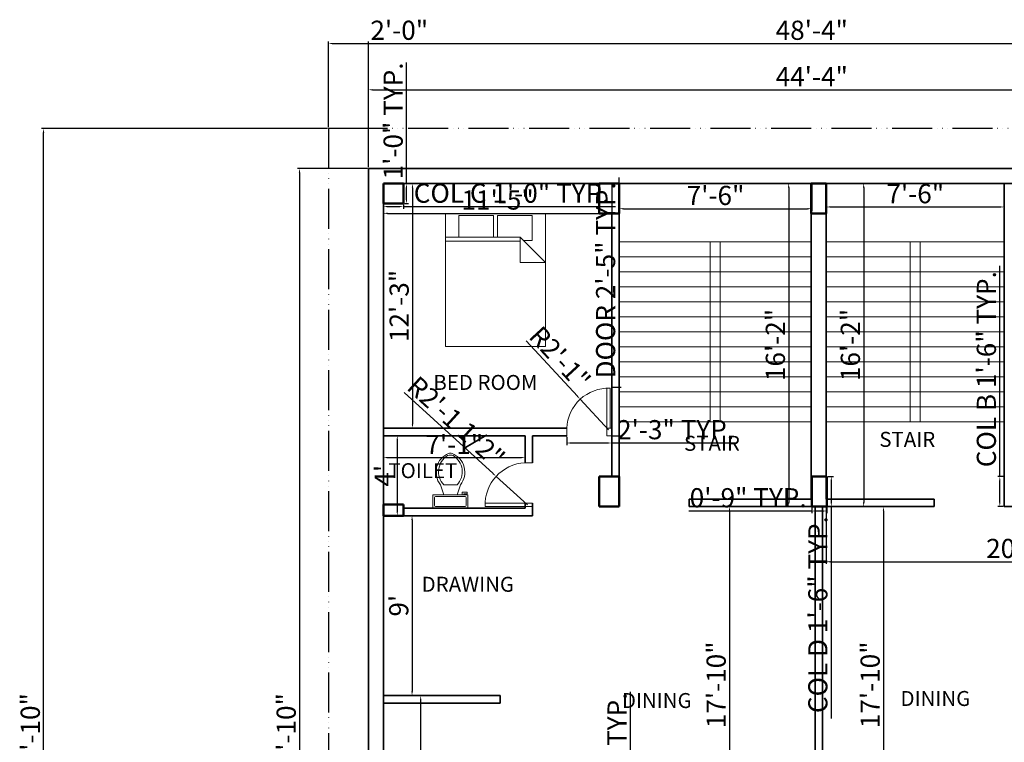
# Model space of a CAD drawing. Units: inches. Extents: x 2680 to 3617, y 1720 to 2823.
# Tile 3 of 4: x 2680 to 3270, y 2380 to 2814. Entities that reach past the tile are written whole.
import ezdxf

# ---------------------------------------------------------------- set-up
doc = ezdxf.new("R2010")
doc.units = ezdxf.units.IN
doc.linetypes.add('ACAD_ISO06W100', pattern=[36, 24, -3, 0, -3, 0, -3, 0, -3])
for name, color, linetype, lineweight in [('A-ANNO-DIMS', 2, 'Continuous', 18), ('A-AREA-IDEN', 244, 'Continuous', 18), ('A-COLS', 1, 'Continuous', 50), ('A-DOOR', 4, 'Continuous', 18), ('A-FLOR-FIXT', 9, 'Continuous', 18), ('A-FLOR-STRS', 7, 'Continuous', 18), ('A-FURN', 8, 'Continuous', 18), ('A-WALL', 7, 'Continuous', 35), ('C-PROP', 6, 'ACAD_ISO06W100', 25)]:
    doc.layers.add(name, color=color, linetype=linetype, lineweight=lineweight)
doc.styles.get("Standard").update_dxf_attribs({"font": 'arial.ttf'})
doc.dimstyles.new('ISO-25', dxfattribs={"dimtxt": 11.5, "dimasz": 2.5, "dimexe": 1.25, "dimexo": 0.625, "dimtad": 1, "dimdec": 1, "dimlunit": 3, "dimtxsty": 'Standard', "dimcen": 2.5, "dimadec": 0, "dimazin": 0, "dimtfac": 1, "dimtdec": 1, "dimtmove": 0, "dimatfit": 3, "dimfxl": 1, "dimarcsym": 0})

# ---------------------------------------------------------------- blocks, each defined once
blk = doc.blocks.new('*D2')
at = {"layer": 'A-ANNO-DIMS', "color": 0, "lineweight": -2, "transparency": 16777216}
for p, q in [((2898.54, 2715.34), (2916.59, 2715.34)), ((2915.34, 2712.84), (2915.34, 2571)), ((2898.54, 2568.5), (2916.59, 2568.5))]:
    blk.add_line(p, q, dxfattribs=at)
at = {"layer": 'A-ANNO-DIMS', "color": 0, "lineweight": 70, "transparency": 16777216}
for points in [[(2914.92, 2712.84), (2915.76, 2712.84), (2915.34, 2715.34)], [(2914.92, 2571), (2915.76, 2571), (2915.34, 2568.5)]]:
    blk.add_solid(points, dxfattribs=at)
at = {"layer": 'Defpoints', "color": 0, "lineweight": 70, "transparency": 16777216}
for p in [(2897.91, 2715.34), (2897.91, 2568.5), (2915.34, 2568.5)]:
    blk.add_point(p, dxfattribs=at)
at = {"layer": 'A-ANNO-DIMS', "color": 0, "transparency": 16777216, "insert": (2908.84, 2641.92), "char_height": 11.5, "attachment_point": 5, "rotation": 90}
blk.add_mtext('12\'-3"', dxfattribs=at)
blk = doc.blocks.new('*D3')
at = {"layer": 'A-ANNO-DIMS', "color": 0, "lineweight": -2, "transparency": 16777216}
for p, q in [((2897.91, 2714.88), (2897.91, 2696.25)), ((3034.91, 2714.88), (3034.91, 2696.25)), ((2900.41, 2697.5), (3032.41, 2697.5))]:
    blk.add_line(p, q, dxfattribs=at)
at = {"layer": 'A-ANNO-DIMS', "color": 0, "lineweight": 70, "transparency": 16777216}
for points in [[(2900.41, 2697.92), (2900.41, 2697.09), (2897.91, 2697.5)], [(3032.41, 2697.92), (3032.41, 2697.09), (3034.91, 2697.5)]]:
    blk.add_solid(points, dxfattribs=at)
at = {"layer": 'Defpoints', "color": 0, "lineweight": 70, "transparency": 16777216}
for p in [(2897.91, 2715.5), (3034.91, 2715.5), (3034.91, 2697.5)]:
    blk.add_point(p, dxfattribs=at)
at = {"layer": 'A-ANNO-DIMS', "color": 0, "transparency": 16777216, "insert": (2966.41, 2704), "char_height": 11.5, "attachment_point": 5}
blk.add_mtext('11\'-5"', dxfattribs=at)
blk = doc.blocks.new('*D4')
at = {"layer": 'A-ANNO-DIMS', "color": 0, "lineweight": -2, "transparency": 16777216}
for p, q in [((3039.41, 2714.88), (3039.41, 2699.02)), ((3154.91, 2714.88), (3154.91, 2699.02)), ((3041.91, 2700.27), (3152.41, 2700.27))]:
    blk.add_line(p, q, dxfattribs=at)
at = {"layer": 'A-ANNO-DIMS', "color": 0, "lineweight": 70, "transparency": 16777216}
for points in [[(3041.91, 2700.68), (3041.91, 2699.85), (3039.41, 2700.27)], [(3152.41, 2700.68), (3152.41, 2699.85), (3154.91, 2700.27)]]:
    blk.add_solid(points, dxfattribs=at)
at = {"layer": 'Defpoints', "color": 0, "lineweight": 70, "transparency": 16777216}
for p in [(3039.41, 2715.5), (3154.91, 2715.5), (3154.91, 2700.27)]:
    blk.add_point(p, dxfattribs=at)
at = {"layer": 'A-ANNO-DIMS', "color": 0, "transparency": 16777216, "insert": (3097.16, 2706.76), "char_height": 11.5, "attachment_point": 5}
blk.add_mtext('7\'-6"', dxfattribs=at)
blk = doc.blocks.new('*D5')
at = {"layer": 'A-ANNO-DIMS', "color": 0, "lineweight": -2, "transparency": 16777216}
for p, q in [((3163.61, 2714.88), (3163.61, 2700.07)), ((3270.41, 2714.8), (3270.41, 2700.07)), ((3166.11, 2701.32), (3267.91, 2701.32))]:
    blk.add_line(p, q, dxfattribs=at)
at = {"layer": 'A-ANNO-DIMS', "color": 0, "lineweight": 70, "transparency": 16777216}
for points in [[(3166.11, 2701.74), (3166.11, 2700.91), (3163.61, 2701.32)], [(3267.91, 2701.74), (3267.91, 2700.91), (3270.41, 2701.32)]]:
    blk.add_solid(points, dxfattribs=at)
at = {"layer": 'Defpoints', "color": 0, "lineweight": 70, "transparency": 16777216}
for p in [(3163.61, 2715.5), (3270.41, 2715.43), (3270.41, 2701.32)]:
    blk.add_point(p, dxfattribs=at)
at = {"layer": 'A-ANNO-DIMS', "color": 0, "transparency": 16777216, "insert": (3217.01, 2707.82), "char_height": 11.5, "width": 83.0724, "attachment_point": 5}
blk.add_mtext('7\'-6"', dxfattribs=at)
blk = doc.blocks.new('*D6')
at = {"layer": 'A-ANNO-DIMS', "color": 0, "lineweight": -2, "transparency": 16777216}
for p, q in [((3154.29, 2715.5), (3139.79, 2715.5)), ((3141.04, 2713), (3141.04, 2524)), ((3154.29, 2521.5), (3139.79, 2521.5))]:
    blk.add_line(p, q, dxfattribs=at)
at = {"layer": 'A-ANNO-DIMS', "color": 0, "lineweight": 70, "transparency": 16777216}
for points in [[(3140.62, 2713), (3141.46, 2713), (3141.04, 2715.5)], [(3140.62, 2524), (3141.46, 2524), (3141.04, 2521.5)]]:
    blk.add_solid(points, dxfattribs=at)
at = {"layer": 'Defpoints', "color": 0, "lineweight": 70, "transparency": 16777216}
for p in [(3154.91, 2715.5), (3141.04, 2521.5), (3154.91, 2521.5)]:
    blk.add_point(p, dxfattribs=at)
at = {"layer": 'A-ANNO-DIMS', "color": 0, "transparency": 16777216, "insert": (3134.54, 2618.5), "char_height": 11.5, "attachment_point": 5, "rotation": 90}
blk.add_mtext('16\'-2"', dxfattribs=at)
blk = doc.blocks.new('*D7')
at = {"layer": 'A-ANNO-DIMS', "color": 0, "lineweight": -2, "transparency": 16777216}
for p, q in [((3164.24, 2715.5), (3187.29, 2715.5)), ((3186.04, 2713), (3186.04, 2524)), ((3164.24, 2521.5), (3187.29, 2521.5))]:
    blk.add_line(p, q, dxfattribs=at)
at = {"layer": 'A-ANNO-DIMS', "color": 0, "lineweight": 70, "transparency": 16777216}
for points in [[(3185.62, 2713), (3186.45, 2713), (3186.04, 2715.5)], [(3185.62, 2524), (3186.45, 2524), (3186.04, 2521.5)]]:
    blk.add_solid(points, dxfattribs=at)
at = {"layer": 'Defpoints', "color": 0, "lineweight": 70, "transparency": 16777216}
for p in [(3163.61, 2715.5), (3163.61, 2521.5), (3186.04, 2521.5)]:
    blk.add_point(p, dxfattribs=at)
at = {"layer": 'A-ANNO-DIMS', "color": 0, "transparency": 16777216, "insert": (3179.54, 2618.5), "char_height": 11.5, "attachment_point": 5, "rotation": 90}
blk.add_mtext('16\'-2"', dxfattribs=at)
blk = doc.blocks.new('*D10')
at = {"layer": 'A-ANNO-DIMS', "color": 0, "lineweight": -2, "transparency": 16777216}
for p, q in [((2897.91, 2563.38), (2897.91, 2549.63)), ((2982.91, 2563.38), (2982.91, 2549.63)), ((2900.41, 2550.88), (2980.41, 2550.88))]:
    blk.add_line(p, q, dxfattribs=at)
at = {"layer": 'A-ANNO-DIMS', "color": 0, "lineweight": 70, "transparency": 16777216}
for points in [[(2900.41, 2551.3), (2900.41, 2550.46), (2897.91, 2550.88)], [(2980.41, 2551.3), (2980.41, 2550.46), (2982.91, 2550.88)]]:
    blk.add_solid(points, dxfattribs=at)
at = {"layer": 'Defpoints', "color": 0, "lineweight": 70, "transparency": 16777216}
for p in [(2897.91, 2564), (2982.91, 2564), (2982.91, 2550.88)]:
    blk.add_point(p, dxfattribs=at)
at = {"layer": 'A-ANNO-DIMS', "color": 0, "transparency": 16777216, "insert": (2940.41, 2557.28), "char_height": 11.5, "attachment_point": 5}
blk.add_mtext('7\'-1"', dxfattribs=at)
blk = doc.blocks.new('*D11')
at = {"layer": 'A-ANNO-DIMS', "color": 0, "lineweight": -2, "transparency": 16777216}
for p, q in [((2898.54, 2564), (2907.47, 2564)), ((2906.22, 2561.5), (2906.22, 2518.5)), ((2898.54, 2516), (2907.47, 2516))]:
    blk.add_line(p, q, dxfattribs=at)
at = {"layer": 'A-ANNO-DIMS', "color": 0, "lineweight": 70, "transparency": 16777216}
for points in [[(2905.8, 2561.5), (2906.63, 2561.5), (2906.22, 2564)], [(2905.8, 2518.5), (2906.63, 2518.5), (2906.22, 2516)]]:
    blk.add_solid(points, dxfattribs=at)
at = {"layer": 'Defpoints', "color": 0, "lineweight": 70, "transparency": 16777216}
for p in [(2897.91, 2564), (2897.91, 2516), (2906.22, 2516)]:
    blk.add_point(p, dxfattribs=at)
at = {"layer": 'A-ANNO-DIMS', "color": 0, "transparency": 16777216, "insert": (2899.84, 2540), "char_height": 11.5, "attachment_point": 5, "rotation": 90}
blk.add_mtext("4'", dxfattribs=at)
blk = doc.blocks.new('*D15')
at = {"layer": 'A-ANNO-DIMS', "color": 0, "lineweight": -2, "transparency": 16777216}
for p, q in [((2898.54, 2408), (2921.5, 2408)), ((2920.25, 2405.5), (2920.25, 2305.5)), ((2898.54, 2303), (2921.5, 2303))]:
    blk.add_line(p, q, dxfattribs=at)
at = {"layer": 'A-ANNO-DIMS', "color": 0, "lineweight": 70, "transparency": 16777216}
for points in [[(2919.83, 2405.5), (2920.66, 2405.5), (2920.25, 2408)], [(2919.83, 2305.5), (2920.66, 2305.5), (2920.25, 2303)]]:
    blk.add_solid(points, dxfattribs=at)
at = {"layer": 'Defpoints', "color": 0, "lineweight": 70, "transparency": 16777216}
for p in [(2897.91, 2408), (2897.91, 2303), (2920.25, 2303)]:
    blk.add_point(p, dxfattribs=at)
at = {"layer": 'A-ANNO-DIMS', "color": 0, "transparency": 16777216, "insert": (2913.75, 2355.5), "char_height": 11.5, "width": 30.5856, "attachment_point": 5, "rotation": 90}
blk.add_mtext('8\'-0"', dxfattribs=at)
blk = doc.blocks.new('*D16')
at = {"layer": 'A-ANNO-DIMS', "color": 0, "lineweight": -2, "transparency": 16777216}
for p, q in [((2898.54, 2516), (2916.34, 2516)), ((2915.09, 2513.5), (2915.09, 2410.5)), ((2898.54, 2408), (2916.34, 2408))]:
    blk.add_line(p, q, dxfattribs=at)
at = {"layer": 'A-ANNO-DIMS', "color": 0, "lineweight": 70, "transparency": 16777216}
for points in [[(2914.67, 2513.5), (2915.5, 2513.5), (2915.09, 2516)], [(2914.67, 2410.5), (2915.5, 2410.5), (2915.09, 2408)]]:
    blk.add_solid(points, dxfattribs=at)
at = {"layer": 'Defpoints', "color": 0, "lineweight": 70, "transparency": 16777216}
for p in [(2897.91, 2516), (2897.91, 2408), (2915.09, 2408)]:
    blk.add_point(p, dxfattribs=at)
at = {"layer": 'A-ANNO-DIMS', "color": 0, "transparency": 16777216, "insert": (2908.59, 2462), "char_height": 11.5, "attachment_point": 5, "rotation": 90}
blk.add_mtext("9'", dxfattribs=at)
blk = doc.blocks.new('*D25')
at = {"layer": 'A-ANNO-DIMS', "color": 0, "lineweight": -2, "transparency": 16777216}
for p, q in [((3082.04, 2521.5), (3106.78, 2521.5)), ((3105.53, 2519), (3105.53, 2310)), ((3084.49, 2307.5), (3106.78, 2307.5))]:
    blk.add_line(p, q, dxfattribs=at)
at = {"layer": 'A-ANNO-DIMS', "color": 0, "lineweight": 70, "transparency": 16777216}
for points in [[(3105.11, 2519), (3105.94, 2519), (3105.53, 2521.5)], [(3105.11, 2310), (3105.94, 2310), (3105.53, 2307.5)]]:
    blk.add_solid(points, dxfattribs=at)
at = {"layer": 'Defpoints', "color": 0, "lineweight": 70, "transparency": 16777216}
for p in [(3081.41, 2521.5), (3083.86, 2307.5), (3105.53, 2307.5)]:
    blk.add_point(p, dxfattribs=at)
at = {"layer": 'A-ANNO-DIMS', "color": 0, "transparency": 16777216, "insert": (3099.03, 2414.5), "char_height": 11.5, "attachment_point": 5, "rotation": 90}
blk.add_mtext('17\'-10"', dxfattribs=at)
blk = doc.blocks.new('*D26')
at = {"layer": 'A-ANNO-DIMS', "color": 0, "lineweight": -2, "transparency": 16777216}
for p, q in [((3227.79, 2521.5), (3196.65, 2521.5)), ((3197.9, 2519), (3197.9, 2310)), ((3226.7, 2307.5), (3196.65, 2307.5))]:
    blk.add_line(p, q, dxfattribs=at)
at = {"layer": 'A-ANNO-DIMS', "color": 0, "lineweight": 70, "transparency": 16777216}
for points in [[(3197.48, 2519), (3198.31, 2519), (3197.9, 2521.5)], [(3197.48, 2310), (3198.31, 2310), (3197.9, 2307.5)]]:
    blk.add_solid(points, dxfattribs=at)
at = {"layer": 'Defpoints', "color": 0, "lineweight": 70, "transparency": 16777216}
for p in [(3228.41, 2521.5), (3197.9, 2307.5), (3227.32, 2307.5)]:
    blk.add_point(p, dxfattribs=at)
at = {"layer": 'A-ANNO-DIMS', "color": 0, "transparency": 16777216, "insert": (3191.4, 2414.5), "char_height": 11.5, "attachment_point": 5, "rotation": 90}
blk.add_mtext('17\'-10"', dxfattribs=at)
blk = doc.blocks.new('*D27')
at = {"layer": 'A-ANNO-DIMS', "color": 0, "lineweight": -2, "transparency": 16777216}
for p, q in [((3163.61, 2520.88), (3163.61, 2487.12)), ((3411.91, 2517.52), (3411.91, 2487.12)), ((3166.11, 2488.37), (3409.41, 2488.37))]:
    blk.add_line(p, q, dxfattribs=at)
at = {"layer": 'A-ANNO-DIMS', "color": 0, "lineweight": 70, "transparency": 16777216}
for points in [[(3166.11, 2488.78), (3166.11, 2487.95), (3163.61, 2488.37)], [(3409.41, 2488.78), (3409.41, 2487.95), (3411.91, 2488.37)]]:
    blk.add_solid(points, dxfattribs=at)
at = {"layer": 'Defpoints', "color": 0, "lineweight": 70, "transparency": 16777216}
for p in [(3163.61, 2521.5), (3411.91, 2518.15), (3411.91, 2488.37)]:
    blk.add_point(p, dxfattribs=at)
at = {"layer": 'A-ANNO-DIMS', "color": 0, "transparency": 16777216, "insert": (3287.76, 2494.87), "char_height": 11.5, "attachment_point": 5}
blk.add_mtext('20\'-8.3"', dxfattribs=at)
blk = doc.blocks.new('*D41')
at = {"layer": 'A-ANNO-DIMS', "color": 0, "lineweight": -2, "transparency": 16777216}
for p, q in [((2888.91, 2725.13), (2888.91, 2772.91)), ((2891.41, 2771.66), (3418.41, 2771.66)), ((3420.91, 2725.13), (3420.91, 2772.91))]:
    blk.add_line(p, q, dxfattribs=at)
at = {"layer": 'A-ANNO-DIMS', "color": 0, "lineweight": 70, "transparency": 16777216}
for points in [[(2891.41, 2772.07), (2891.41, 2771.24), (2888.91, 2771.66)], [(3418.41, 2772.07), (3418.41, 2771.24), (3420.91, 2771.66)]]:
    blk.add_solid(points, dxfattribs=at)
at = {"layer": 'Defpoints', "color": 0, "lineweight": 70, "transparency": 16777216}
for p in [(3420.91, 2771.66), (2888.91, 2724.5), (3420.91, 2724.5)]:
    blk.add_point(p, dxfattribs=at)
at = {"layer": 'A-ANNO-DIMS', "color": 0, "transparency": 16777216, "insert": (3154.91, 2778.03), "char_height": 11.5, "attachment_point": 5}
blk.add_mtext('44\'-4"', dxfattribs=at)
blk = doc.blocks.new('*D42')
at = {"layer": 'A-ANNO-DIMS', "color": 0, "lineweight": -2, "transparency": 16777216}
for p, q in [((2888.29, 2724.5), (2846.31, 2724.5)), ((2847.56, 2722), (2847.56, 2045)), ((2888.29, 2042.5), (2846.31, 2042.5))]:
    blk.add_line(p, q, dxfattribs=at)
at = {"layer": 'A-ANNO-DIMS', "color": 0, "lineweight": 70, "transparency": 16777216}
for points in [[(2847.14, 2722), (2847.98, 2722), (2847.56, 2724.5)], [(2847.14, 2045), (2847.98, 2045), (2847.56, 2042.5)]]:
    blk.add_solid(points, dxfattribs=at)
at = {"layer": 'Defpoints', "color": 0, "lineweight": 70, "transparency": 16777216}
for p in [(2888.91, 2724.5), (2847.56, 2042.5), (2888.91, 2042.5)]:
    blk.add_point(p, dxfattribs=at)
at = {"layer": 'A-ANNO-DIMS', "color": 0, "transparency": 16777216, "insert": (2841.06, 2383.5), "char_height": 11.5, "attachment_point": 5, "rotation": 90}
blk.add_mtext('56\'-10"', dxfattribs=at)
blk = doc.blocks.new('Bed - Queen')
for p, q in [((0, -80.00003), (0, 0)), ((0, 0), (59.99999, 0)), ((59.99999, 0), (59.99999, -80.00003)), ((7.99999, -1.2), (28.79998, -1.2)), ((7.99999, -14.4), (7.99999, -1.2)), ((28.79998, -1.2), (28.79998, -14.4)), ((31.19999, -1.2), (51.99999, -1.2)), ((31.19999, -14.4), (31.19999, -1.2)), ((51.99999, -1.2), (51.99999, -16.4)), ((0, -14.4), (44.8, -14.4)), ((44.8, -16.8), (0, -16.8)), ((59.99999, -29.6), (44.8, -14.4)), ((44.8, -14.4), (44.8, -29.6)), ((51.99999, -16.4), (46.79936, -16.4)), ((44.8, -29.6), (59.99999, -29.6)), ((59.99999, -80.00003), (0, -80.00003))]:
    blk.add_line(p, q)
blk = doc.blocks.new('Toilet - top')
for p, q in [((9.5, -6), (9.5, -2)), ((-10, -8.5), (-8, -8.5)), ((-10, -9.5), (-10, -8.5)), ((-7, -9.5), (-10, -9.5)), ((-8, -8.5), (-8, -8)), ((-7, -8), (-7, -9.5)), ((-4, -8), (-6, -14)), ((4, -8), (6, -14)), ((4, -14), (-4, -14))]:
    blk.add_line(p, q)
blk.add_lwpolyline([(10.5, -8), (10.5, 0), (-10.5, 0), (-10.5, -8)], close=True)
for points in [[(-9.5, -2), (-9.5, -6)], [(8.5, -1), (-8.5, -1)], [(-8.5, -7), (8.5, -7)]]:
    blk.add_lwpolyline(points)
for centre, radius, start, end in [((-8.62, -1.88), 0.884, 81.8699, 188.1301), ((8.62, -1.88), 0.884, 351.8699, 98.1301), ((-8.62, -6.12), 0.884, 171.8699, 278.1301), ((8.62, -6.12), 0.884, 261.8699, 8.1301), ((3.52, -21.58), 12.17, 141.46911, 247.97143), ((4.2, -21.82), 11.33, 136.36773, 238.94682), ((-3.52, -21.58), 12.17, 292.02843, 38.53071), ((-4.2, -21.82), 11.33, 301.05301, 43.63209), ((0, -27.88), 4, 245.73182, 294.26817), ((0, -29), 4, 254.86053, 285.13947)]:
    blk.add_arc(centre, radius, start, end)
blk = doc.blocks.new('COL-12X6P64')
for p, q in [((0, 0), (0, 6.64)), ((0, 6.64), (12, 6.64)), ((12, 6.64), (12, 0)), ((12, 0), (0, 0))]:
    blk.add_line(p, q)
blk = doc.blocks.new('COL-12X18')
for p, q in [((0, 0), (0, 18)), ((0, 18), (12, 18)), ((12, 18), (12, 0)), ((12, 18), (12, 0)), ((12, 0), (0, 0))]:
    blk.add_line(p, q)
blk = doc.blocks.new('COL-12X12')
for p, q in [((0, 12), (12, 12)), ((0, 0), (0, 12)), ((12, 12), (12, 0)), ((12, 0), (0, 0))]:
    blk.add_line(p, q)
blk = doc.blocks.new('COL-9X18')
for p, q in [((9, 18), (0, 18)), ((0, 18), (0, 0)), ((9, 0), (9, 18)), ((0, 0), (9, 0))]:
    blk.add_line(p, q)
blk = doc.blocks.new('DOOR-SINGLE-27')
for p, q in [((26, 28.5), (24, 28.5)), ((24, 28.5), (24, 0)), ((26, 4.5), (26, 28.5)), ((0, 4.5), (0, 0)), ((24, 4.5), (27, 4.5)), ((27, 4.5), (26, 4.5)), ((24, 0), (27, 0))]:
    blk.add_line(p, q)
blk.add_arc((25, 3.5), 25.02, 87.70939, 177.70939)
blk = doc.blocks.new('*D59')
at = {"layer": 'A-ANNO-DIMS', "color": 0, "lineweight": -2, "transparency": 16777216}
for p, q in [((3046.11, 2309.65), (3046.11, 2410.29)), ((3044.93, 2309.65), (3047.36, 2309.65)), ((3046.11, 2305.5), (3046.11, 2307.15)), ((3044.93, 2303), (3047.36, 2303))]:
    blk.add_line(p, q, dxfattribs=at)
at = {"layer": 'A-ANNO-DIMS', "color": 0, "lineweight": 70, "transparency": 16777216}
for points in [[(3045.69, 2307.15), (3046.52, 2307.15), (3046.11, 2309.65)], [(3045.69, 2305.5), (3046.52, 2305.5), (3046.11, 2303)]]:
    blk.add_solid(points, dxfattribs=at)
at = {"layer": 'Defpoints', "color": 0, "lineweight": 70, "transparency": 16777216}
for p in [(3044.31, 2309.65), (3046.11, 2309.65), (3044.31, 2303)]:
    blk.add_point(p, dxfattribs=at)
at = {"layer": 'A-ANNO-DIMS', "color": 0, "transparency": 16777216, "insert": (3039.54, 2361.22), "char_height": 11.5, "attachment_point": 5, "rotation": 90}
blk.add_mtext('0\'-6 1/2" TYP.', dxfattribs=at)
blk = doc.blocks.new('*D60')
at = {"layer": 'A-ANNO-DIMS', "color": 0, "lineweight": -2, "transparency": 16777216}
for p, q in [((3267.71, 2539.5), (3267.71, 2665.89)), ((3269.79, 2539.5), (3266.46, 2539.5)), ((3267.71, 2524), (3267.71, 2537)), ((3269.79, 2521.5), (3266.46, 2521.5))]:
    blk.add_line(p, q, dxfattribs=at)
at = {"layer": 'A-ANNO-DIMS', "color": 0, "lineweight": 70, "transparency": 16777216}
for points in [[(3267.3, 2537), (3268.13, 2537), (3267.71, 2539.5)], [(3267.3, 2524), (3268.13, 2524), (3267.71, 2521.5)]]:
    blk.add_solid(points, dxfattribs=at)
at = {"layer": 'Defpoints', "color": 0, "lineweight": 70, "transparency": 16777216}
for p in [(3267.71, 2539.5), (3270.41, 2539.5), (3270.41, 2521.5)]:
    blk.add_point(p, dxfattribs=at)
at = {"layer": 'A-ANNO-DIMS', "color": 0, "transparency": 16777216, "insert": (3261.14, 2603.95), "char_height": 11.5, "attachment_point": 5, "rotation": 90}
blk.add_mtext('COL B 1\'-6" TYP.', dxfattribs=at)
blk = doc.blocks.new('*D62')
at = {"layer": 'A-ANNO-DIMS', "color": 0, "lineweight": -2, "transparency": 16777216}
for p, q in [((2897.91, 2702.71), (2897.91, 2700.29)), ((2900.41, 2701.54), (2907.41, 2701.54)), ((2909.91, 2702.71), (2909.91, 2700.29)), ((2909.91, 2701.54), (3037.19, 2701.54))]:
    blk.add_line(p, q, dxfattribs=at)
at = {"layer": 'A-ANNO-DIMS', "color": 0, "lineweight": 70, "transparency": 16777216}
for points in [[(2900.41, 2701.95), (2900.41, 2701.12), (2897.91, 2701.54)], [(2907.41, 2701.95), (2907.41, 2701.12), (2909.91, 2701.54)]]:
    blk.add_solid(points, dxfattribs=at)
at = {"layer": 'Defpoints', "color": 0, "lineweight": 70, "transparency": 16777216}
for p in [(2897.91, 2703.34), (2909.91, 2703.34), (2909.91, 2701.54)]:
    blk.add_point(p, dxfattribs=at)
at = {"layer": 'A-ANNO-DIMS', "color": 0, "transparency": 16777216, "insert": (2974.8, 2708.11), "char_height": 11.5, "attachment_point": 5}
blk.add_mtext('COL C 1\'-0" TYP.', dxfattribs=at)
blk = doc.blocks.new('*D63')
at = {"layer": 'A-ANNO-DIMS', "color": 0, "lineweight": -2, "transparency": 16777216}
for p, q in [((2911.71, 2715.34), (2911.71, 2788.1)), ((2910.54, 2715.34), (2912.96, 2715.34)), ((2911.71, 2705.84), (2911.71, 2712.84)), ((2910.54, 2703.34), (2912.96, 2703.34))]:
    blk.add_line(p, q, dxfattribs=at)
at = {"layer": 'A-ANNO-DIMS', "color": 0, "lineweight": 70, "transparency": 16777216}
for points in [[(2911.3, 2712.84), (2912.13, 2712.84), (2911.71, 2715.34)], [(2911.3, 2705.84), (2912.13, 2705.84), (2911.71, 2703.34)]]:
    blk.add_solid(points, dxfattribs=at)
at = {"layer": 'Defpoints', "color": 0, "lineweight": 70, "transparency": 16777216}
for p in [(2909.91, 2715.34), (2911.71, 2715.34), (2909.91, 2703.34)]:
    blk.add_point(p, dxfattribs=at)
at = {"layer": 'A-ANNO-DIMS', "color": 0, "transparency": 16777216, "insert": (2905.22, 2752.97), "char_height": 11.5, "attachment_point": 5, "rotation": 90}
blk.add_mtext('1\'-0" TYP.', dxfattribs=at)
blk = doc.blocks.new('*D64')
at = {"layer": 'A-ANNO-DIMS', "color": 0, "lineweight": -2, "transparency": 16777216}
for p, q in [((3164.54, 2539.5), (3167.86, 2539.5)), ((3166.61, 2537), (3166.61, 2524)), ((3164.54, 2521.5), (3167.86, 2521.5)), ((3166.61, 2521.5), (3166.61, 2394.23))]:
    blk.add_line(p, q, dxfattribs=at)
at = {"layer": 'A-ANNO-DIMS', "color": 0, "lineweight": 70, "transparency": 16777216}
for points in [[(3166.2, 2537), (3167.03, 2537), (3166.61, 2539.5)], [(3166.2, 2524), (3167.03, 2524), (3166.61, 2521.5)]]:
    blk.add_solid(points, dxfattribs=at)
at = {"layer": 'Defpoints', "color": 0, "lineweight": 70, "transparency": 16777216}
for p in [(3163.91, 2539.5), (3163.91, 2521.5), (3166.61, 2521.5)]:
    blk.add_point(p, dxfattribs=at)
at = {"layer": 'A-ANNO-DIMS', "color": 0, "transparency": 16777216, "insert": (3160.04, 2456.62), "char_height": 11.5, "attachment_point": 5, "rotation": 90}
blk.add_mtext('COL D 1\'-6" TYP.', dxfattribs=at)
blk = doc.blocks.new('*D65')
at = {"layer": 'A-ANNO-DIMS', "color": 0, "lineweight": -2, "transparency": 16777216}
for p, q in [((3154.91, 2518.8), (3081.07, 2518.8)), ((3154.91, 2520.88), (3154.91, 2517.55)), ((3161.41, 2518.8), (3157.41, 2518.8)), ((3163.91, 2520.88), (3163.91, 2517.55))]:
    blk.add_line(p, q, dxfattribs=at)
at = {"layer": 'A-ANNO-DIMS', "color": 0, "lineweight": 70, "transparency": 16777216}
for points in [[(3157.41, 2519.22), (3157.41, 2518.39), (3154.91, 2518.8)], [(3161.41, 2519.22), (3161.41, 2518.39), (3163.91, 2518.8)]]:
    blk.add_solid(points, dxfattribs=at)
at = {"layer": 'Defpoints', "color": 0, "lineweight": 70, "transparency": 16777216}
for p in [(3154.91, 2521.5), (3154.91, 2518.8), (3163.91, 2521.5)]:
    blk.add_point(p, dxfattribs=at)
at = {"layer": 'A-ANNO-DIMS', "color": 0, "transparency": 16777216, "insert": (3116.74, 2525.3), "char_height": 11.5, "attachment_point": 5}
blk.add_mtext('0\'-9" TYP.', dxfattribs=at)
blk = doc.blocks.new('*D66')
at = {"layer": 'A-ANNO-DIMS', "color": 0, "lineweight": -2, "transparency": 16777216}
for p, q in [((3039.27, 2593.06), (3039.27, 2718.99)), ((3035.54, 2593.06), (3040.52, 2593.06)), ((3039.27, 2566.5), (3039.27, 2590.56)), ((3035.54, 2564), (3040.52, 2564))]:
    blk.add_line(p, q, dxfattribs=at)
at = {"layer": 'A-ANNO-DIMS', "color": 0, "lineweight": 70, "transparency": 16777216}
for points in [[(3038.86, 2590.56), (3039.69, 2590.56), (3039.27, 2593.06)], [(3038.86, 2566.5), (3039.69, 2566.5), (3039.27, 2564)]]:
    blk.add_solid(points, dxfattribs=at)
at = {"layer": 'Defpoints', "color": 0, "lineweight": 70, "transparency": 16777216}
for p in [(3034.91, 2593.06), (3039.27, 2593.06), (3034.91, 2564)]:
    blk.add_point(p, dxfattribs=at)
at = {"layer": 'A-ANNO-DIMS', "color": 0, "transparency": 16777216, "insert": (3032.7, 2657.27), "char_height": 11.5, "attachment_point": 5, "rotation": 90}
blk.add_mtext('DOOR 2\'-5" TYP.', dxfattribs=at)
blk = doc.blocks.new('*D67')
at = {"layer": 'A-ANNO-DIMS', "color": 0, "lineweight": -2, "transparency": 16777216}
for p, q in [((3007.91, 2563.38), (3007.91, 2558.4)), ((3010.41, 2559.65), (3032.41, 2559.65)), ((3034.91, 2563.38), (3034.91, 2558.4)), ((3034.91, 2559.65), (3108.96, 2559.65))]:
    blk.add_line(p, q, dxfattribs=at)
at = {"layer": 'A-ANNO-DIMS', "color": 0, "lineweight": 70, "transparency": 16777216}
for points in [[(3010.41, 2560.06), (3010.41, 2559.23), (3007.91, 2559.65)], [(3032.41, 2560.06), (3032.41, 2559.23), (3034.91, 2559.65)]]:
    blk.add_solid(points, dxfattribs=at)
at = {"layer": 'Defpoints', "color": 0, "lineweight": 70, "transparency": 16777216}
for p in [(3007.91, 2564), (3034.91, 2564), (3034.91, 2559.65)]:
    blk.add_point(p, dxfattribs=at)
at = {"layer": 'A-ANNO-DIMS', "color": 0, "transparency": 16777216, "insert": (3073.19, 2566.15), "char_height": 11.5, "attachment_point": 5}
blk.add_mtext('2\'-3" TYP.', dxfattribs=at)
blk = doc.blocks.new('*D68')
at = {"layer": 'A-ANNO-DIMS', "color": 0, "lineweight": -2, "transparency": 16777216}
for p, q in [((2864.91, 2749.13), (2864.91, 2800.65)), ((3444.91, 2749.13), (3444.91, 2800.65)), ((2867.41, 2799.4), (3442.41, 2799.4))]:
    blk.add_line(p, q, dxfattribs=at)
at = {"layer": 'A-ANNO-DIMS', "color": 0, "lineweight": 70, "transparency": 16777216}
for points in [[(2867.41, 2799.82), (2867.41, 2798.99), (2864.91, 2799.4)], [(3442.41, 2799.82), (3442.41, 2798.99), (3444.91, 2799.4)]]:
    blk.add_solid(points, dxfattribs=at)
at = {"layer": 'Defpoints', "color": 0, "lineweight": 70, "transparency": 16777216}
for p in [(3444.91, 2799.4), (2864.91, 2748.5), (3444.91, 2748.5)]:
    blk.add_point(p, dxfattribs=at)
at = {"layer": 'A-ANNO-DIMS', "color": 0, "transparency": 16777216, "insert": (3154.91, 2805.9), "char_height": 11.5, "attachment_point": 5}
blk.add_mtext('48\'-4"', dxfattribs=at)
blk = doc.blocks.new('*D69')
at = {"layer": 'A-ANNO-DIMS', "color": 0, "lineweight": -2, "transparency": 16777216}
for p, q in [((2864.29, 2748.5), (2692.76, 2748.5)), ((2694.01, 2021), (2694.01, 2746)), ((2864.29, 2018.5), (2692.76, 2018.5))]:
    blk.add_line(p, q, dxfattribs=at)
at = {"layer": 'A-ANNO-DIMS', "color": 0, "lineweight": 70, "transparency": 16777216}
for points in [[(2693.6, 2746), (2694.43, 2746), (2694.01, 2748.5)], [(2693.6, 2021), (2694.43, 2021), (2694.01, 2018.5)]]:
    blk.add_solid(points, dxfattribs=at)
at = {"layer": 'Defpoints', "color": 0, "lineweight": 70, "transparency": 16777216}
for p in [(2694.01, 2748.5), (2864.91, 2748.5), (2864.91, 2018.5)]:
    blk.add_point(p, dxfattribs=at)
at = {"layer": 'A-ANNO-DIMS', "color": 0, "transparency": 16777216, "insert": (2687.52, 2383.5), "char_height": 11.5, "attachment_point": 5, "rotation": 90}
blk.add_mtext('60\'-10"', dxfattribs=at)
blk = doc.blocks.new('*D71')
at = {"layer": 'A-ANNO-DIMS', "color": 0, "lineweight": -2, "transparency": 16777216}
for p, q in [((2864.91, 2749.13), (2864.91, 2800.65)), ((2888.91, 2725.13), (2888.91, 2800.65)), ((2867.41, 2799.4), (2886.41, 2799.4)), ((2888.91, 2799.4), (2923.43, 2799.4))]:
    blk.add_line(p, q, dxfattribs=at)
at = {"layer": 'A-ANNO-DIMS', "color": 0, "lineweight": 70, "transparency": 16777216}
for points in [[(2867.41, 2799.82), (2867.41, 2798.99), (2864.91, 2799.4)], [(2886.41, 2799.82), (2886.41, 2798.99), (2888.91, 2799.4)]]:
    blk.add_solid(points, dxfattribs=at)
at = {"layer": 'Defpoints', "color": 0, "lineweight": 70, "transparency": 16777216}
for p in [(2888.91, 2799.4), (2864.91, 2748.5), (2888.91, 2724.5)]:
    blk.add_point(p, dxfattribs=at)
at = {"layer": 'A-ANNO-DIMS', "color": 0, "transparency": 16777216, "insert": (2907.42, 2805.9), "char_height": 11.5, "attachment_point": 5}
blk.add_mtext('2\'-0"', dxfattribs=at)
blk = doc.blocks.new('*D76')
at = {"layer": 'A-ANNO-DIMS', "color": 0, "lineweight": -2, "transparency": 16777216}
for p, q in [((2910.37, 2589.87), (2963.67, 2541.27)), ((2984.25, 2522.5), (2965.51, 2539.59))]:
    blk.add_line(p, q, dxfattribs=at)
at = {"layer": 'A-ANNO-DIMS', "color": 0, "lineweight": 70, "transparency": 16777216}
blk.add_solid([(2963.95, 2541.58), (2963.39, 2540.97), (2965.51, 2539.59)], dxfattribs=at)
at = {"layer": 'Defpoints', "color": 0, "lineweight": 70, "transparency": 16777216}
for p in [(2965.51, 2539.59), (2984.25, 2522.5)]:
    blk.add_point(p, dxfattribs=at)
at = {"layer": 'A-ANNO-DIMS', "color": 0, "transparency": 16777216, "insert": (2940.52, 2571.27), "char_height": 11.5, "attachment_point": 5, "rotation": 317.64247}
blk.add_mtext('R2\'-1 1/2"', dxfattribs=at)
blk = doc.blocks.new('*D77')
at = {"layer": 'A-ANNO-DIMS', "color": 0, "lineweight": -2, "transparency": 16777216}
for p, q in [((2983.51, 2621.03), (3014.25, 2587.73)), ((3032.91, 2567.5), (3015.94, 2585.89))]:
    blk.add_line(p, q, dxfattribs=at)
at = {"layer": 'A-ANNO-DIMS', "color": 0, "lineweight": 70, "transparency": 16777216}
blk.add_solid([(3014.55, 2588.01), (3013.94, 2587.44), (3015.94, 2585.89)], dxfattribs=at)
at = {"layer": 'Defpoints', "color": 0, "lineweight": 70, "transparency": 16777216}
for p in [(3015.94, 2585.89), (3032.91, 2567.5)]:
    blk.add_point(p, dxfattribs=at)
at = {"layer": 'A-ANNO-DIMS', "color": 0, "transparency": 16777216, "insert": (3002.73, 2609.64), "char_height": 11.5, "attachment_point": 5, "rotation": 312.70869}
blk.add_mtext('R2\'-1"', dxfattribs=at)

msp = doc.modelspace()

# ---------------------------------------------------------------- linework, layer by layer
at = {"layer": 'A-DOOR'}
for p, q in [((2982.91, 2547.83), (2987.41, 2547.83)), ((2958.91, 2521.5), (2958.91, 2523.5)), ((2958.91, 2523.5), (2987.41, 2523.5)), ((2982.91, 2521.5), (2958.91, 2521.5)), ((2958.91, 2521.5), (2987.41, 2521.5)), ((2982.91, 2520.5), (2982.91, 2521.5)), ((2982.91, 2520.5), (2982.91, 2520.5))]:
    msp.add_line(p, q, dxfattribs=at)
msp.add_arc((2984.25, 2522.5), 25.36, 93.02461, 182.26009, dxfattribs=at)
at = {"layer": 'A-FLOR-STRS'}
for p, q in [((3039.41, 2680.42), (3154.61, 2680.42)), ((3094.01, 2680.42), (3094.01, 2572.42)), ((3100.01, 2680.42), (3100.01, 2572.42)), ((3163.61, 2680.42), (3270.41, 2680.42)), ((3214.01, 2680.42), (3214.01, 2572.42)), ((3220.01, 2680.42), (3220.01, 2572.42)), ((3039.41, 2671.42), (3154.61, 2671.42)), ((3163.61, 2671.42), (3270.41, 2671.42)), ((3039.41, 2662.42), (3154.61, 2662.42)), ((3163.61, 2662.42), (3270.41, 2662.42)), ((3039.41, 2653.42), (3154.61, 2653.42)), ((3163.61, 2653.42), (3270.41, 2653.42)), ((3039.41, 2644.42), (3154.61, 2644.42)), ((3163.61, 2644.42), (3270.41, 2644.42)), ((3039.41, 2635.42), (3154.61, 2635.42)), ((3163.61, 2635.42), (3270.41, 2635.42)), ((3039.41, 2626.42), (3154.61, 2626.42)), ((3163.61, 2626.42), (3270.41, 2626.42)), ((3039.41, 2617.42), (3154.61, 2617.42)), ((3163.61, 2617.42), (3270.41, 2617.42)), ((3039.41, 2608.42), (3154.61, 2608.42)), ((3163.61, 2608.42), (3270.41, 2608.42)), ((3039.41, 2599.42), (3154.61, 2599.42)), ((3163.61, 2599.42), (3270.41, 2599.42)), ((3039.41, 2590.42), (3154.61, 2590.42)), ((3039.41, 2590.42), (3154.61, 2590.42)), ((3163.61, 2590.42), (3270.41, 2590.42)), ((3163.61, 2590.42), (3270.41, 2590.42)), ((3039.41, 2581.42), (3154.61, 2581.42)), ((3163.61, 2581.42), (3270.41, 2581.42)), ((3039.41, 2572.42), (3154.61, 2572.42)), ((3163.61, 2572.42), (3270.41, 2572.42))]:
    msp.add_line(p, q, dxfattribs=at)
at = {"layer": 'A-WALL'}
for p, q in [((2888.91, 2724.5), (3420.91, 2724.5)), ((2888.91, 2090.5), (2888.91, 2724.5)), ((2897.91, 2715.5), (3411.91, 2715.5)), ((2897.91, 2090.5), (2897.91, 2715.5)), ((3039.41, 2564), (3039.41, 2715.5)), ((3154.61, 2715.5), (3154.61, 2526)), ((3163.61, 2715.5), (3163.61, 2526)), ((3270.41, 2715.5), (3270.41, 2521.5)), ((3034.91, 2564), (3034.91, 2697.5)), ((2897.91, 2568.5), (3007.91, 2568.5)), ((2897.91, 2564), (2982.91, 2564)), ((2982.91, 2547.83), (2982.91, 2564)), ((2987.41, 2564), (3007.91, 2564)), ((2987.41, 2547.83), (2987.41, 2564)), ((3034.91, 2539.51), (3034.91, 2564)), ((3039.41, 2521.5), (3039.41, 2564)), ((2982.91, 2520.5), (2982.91, 2523.5)), ((2987.41, 2516), (2987.41, 2523.5)), ((3081.41, 2521.5), (3081.41, 2526)), ((3081.41, 2526), (3154.61, 2526)), ((3163.61, 2526), (3228.41, 2526)), ((3228.41, 2521.5), (3228.41, 2526)), ((2909.91, 2520.5), (2982.91, 2520.5)), ((3034.91, 2521.5), (3034.91, 2521.51)), ((3039.41, 2521.5), (3034.91, 2521.5)), ((3034.91, 2521.5), (3039.41, 2521.5)), ((3081.41, 2521.5), (3228.41, 2521.5)), ((3156.91, 2521.5), (3156.91, 2042.5)), ((3163.61, 2521.5), (3159.11, 2521.5)), ((3161.31, 2521.5), (3161.31, 2042.5)), ((3270.41, 2521.5), (3274.91, 2521.5)), ((2897.91, 2516), (2987.41, 2516)), ((2897.91, 2408), (2967.91, 2408)), ((2967.91, 2403.5), (2967.91, 2408)), ((2897.91, 2403.5), (2967.91, 2403.5))]:
    msp.add_line(p, q, dxfattribs=at)
at = {"layer": 'C-PROP'}
for p, q in [((2888.91, 2748.5), (2864.91, 2748.5)), ((2864.91, 2748.5), (2864.91, 2042.5)), ((3444.91, 2748.5), (2888.91, 2748.5))]:
    msp.add_line(p, q, dxfattribs=at)

# ---------------------------------------------------------------- block references
at = {"layer": 'A-COLS'}
for name, p in [('COL-12X12', (2897.91, 2703.34)), ('COL-12X18', (3027.41, 2697.5)), ('COL-9X18', (3154.61, 2697.5)), ('COL-12X18', (3027.33, 2521.51)), ('COL-12X6P64', (2897.91, 2516))]:
    msp.add_blockref(name, p, dxfattribs=at)
at = {"layer": 'A-COLS', "rotation": 180}
msp.add_blockref('COL-9X18', (3163.91, 2539.5), dxfattribs=at)
at = {"layer": 'A-DOOR'}
msp.add_blockref('DOOR-SINGLE-27', (3007.91, 2564), dxfattribs=at)
at = {"layer": 'A-FLOR-FIXT', "rotation": 180}
msp.add_blockref('Toilet - top', (2938.09, 2520.54), dxfattribs=at)
at = {"layer": 'A-FURN'}
msp.add_blockref('Bed - Queen', (2935.18, 2697.5), dxfattribs=at)

# ---------------------------------------------------------------- texts
at = {"layer": 'A-AREA-IDEN', "char_height": 9, "attachment_point": 1}
for s, insert in [('{BED ROOM}', (2927.87, 2600.5)), ('{STAIR}', (3078.25, 2563.96)), ('{STAIR}', (3195.43, 2566.31)), ('{TOILET}', (2900.87, 2547.54)), ('{DRAWING}', (2920.83, 2479.35)), ('{DINING}', (3208.15, 2410.79)), ('{DINING}', (3040.98, 2409.56))]:
    msp.add_mtext_dynamic_manual_height_columns(s, width=87.2951, gutter_width=12.5, heights=[0], dxfattribs=dict(at, insert=insert))

# ---------------------------------------------------------------- dimensions: what is measured, and where the dimension line sits
at = {"layer": 'A-ANNO-DIMS'}
for base, p1, p2, override, picture, middle in [((3444.91, 2799.4), (2864.91, 2748.5), (3444.91, 2748.5), {"dimdec": 1, "dimlfac": 1, "dimrnd": 0, "dimzin": 1, "dimdsep": 46, "dimlunit": 4, "dimfrac": 2}, '*D68', (3154.91, 2805.9)), ((2888.91, 2799.4), (2864.91, 2748.5), (2888.91, 2724.5), {"dimdec": 1, "dimlfac": 1, "dimrnd": 0, "dimzin": 1, "dimdsep": 46, "dimlunit": 4, "dimfrac": 2}, '*D71', (2907.42, 2805.9)), ((3420.91, 2771.66), (2888.91, 2724.5), (3420.91, 2724.5), {"dimclrd": 0, "dimclre": 0, "dimclrt": 0}, '*D41', (3154.91, 2778.03)), ((3034.91, 2697.5), (2897.91, 2715.5), (3034.91, 2715.5), {"dimclrd": 0, "dimclre": 0, "dimclrt": 0}, '*D3', (2966.41, 2704)), ((2982.91, 2550.88), (2897.91, 2564), (2982.91, 2564), {"dimclrd": 0, "dimclre": 0, "dimclrt": 0}, '*D10', (2940.41, 2557.28)), ((3411.91, 2488.37), (3163.61, 2521.5), (3411.91, 2518.15), {"dimclrd": 0, "dimclre": 0, "dimclrt": 0}, '*D27', (3287.76, 2494.87))]:
    dim = msp.add_linear_dim(base=base, p1=p1, p2=p2, dimstyle='ISO-25', override=override, dxfattribs=at)
    dim.commit()
    dim.dimension.update_dxf_attribs({"geometry": picture, "text_midpoint": middle})
for base, p1, p2, angle, text, override, picture, middle in [((2911.71, 2715.34), (2909.91, 2703.34), (2909.91, 2715.34), 90, '<> TYP.', {"dimdec": 1, "dimlfac": 1, "dimrnd": 0, "dimzin": 1, "dimdsep": 46, "dimlunit": 4, "dimfrac": 2}, '*D63', (2905.22, 2752.97)), ((3039.27, 2593.06), (3034.91, 2564), (3034.91, 2593.06), 90, 'DOOR <> TYP.', {"dimdec": 1, "dimlfac": 1, "dimrnd": 0, "dimzin": 1, "dimdsep": 46, "dimlunit": 4, "dimfrac": 2}, '*D66', (3032.7, 2657.27)), ((2915.34, 2568.5), (2897.91, 2715.34), (2897.91, 2568.5), 90, '12\'-3"', {"dimclrd": 0, "dimclre": 0, "dimclrt": 0}, '*D2', (2908.84, 2641.92)), ((3267.71, 2539.5), (3270.41, 2521.5), (3270.41, 2539.5), 90, 'COL B <> TYP.', {"dimdec": 1, "dimlfac": 1, "dimrnd": 0, "dimzin": 1, "dimdsep": 46, "dimlunit": 4, "dimfrac": 2}, '*D60', (3261.14, 2603.95)), ((3154.91, 2518.8), (3163.91, 2521.5), (3154.91, 2521.5), 180, '<> TYP.', {"dimdec": 1, "dimlfac": 1, "dimrnd": 0, "dimzin": 1, "dimdsep": 46, "dimlunit": 4, "dimfrac": 2}, '*D65', (3116.74, 2525.3)), ((3166.61, 2521.5), (3163.91, 2539.5), (3163.91, 2521.5), 270, 'COL D <> TYP.', {"dimdec": 1, "dimlfac": 1, "dimrnd": 0, "dimzin": 1, "dimdsep": 46, "dimlunit": 4, "dimfrac": 2}, '*D64', (3160.04, 2456.62)), ((3046.1082, 2309.6469), (3044.3082, 2303.0039), (3044.3082, 2309.6469), 90, '<> TYP.', {"dimdec": 1, "dimlfac": 1, "dimrnd": 0, "dimzin": 1, "dimdsep": 46, "dimlunit": 4, "dimfrac": 2}, '*D59', (3039.5371, 2361.2194)), ((2920.25, 2303), (2897.91, 2408), (2897.91, 2303), 90, '8\'-0"', {"dimclrd": 0, "dimclre": 0, "dimclrt": 0}, '*D15', (2913.75, 2355.5))]:
    dim = msp.add_linear_dim(base=base, p1=p1, p2=p2, angle=angle, text=text, dimstyle='ISO-25', override=override, dxfattribs=at)
    dim.commit()
    dim.dimension.update_dxf_attribs({"geometry": picture, "text_midpoint": middle})
for base, p1, p2, override, picture, middle in [((2694.01, 2748.5), (2864.91, 2018.5), (2864.91, 2748.5), {"dimdec": 1, "dimlfac": 1, "dimrnd": 0, "dimzin": 1, "dimdsep": 46, "dimlunit": 4, "dimfrac": 2}, '*D69', (2687.52, 2383.5)), ((2847.56, 2042.5), (2888.91, 2724.5), (2888.91, 2042.5), {"dimclrd": 0, "dimclre": 0, "dimclrt": 0}, '*D42', (2841.06, 2383.5)), ((3141.04, 2521.5), (3154.91, 2715.5), (3154.91, 2521.5), {"dimclrd": 0, "dimclre": 0, "dimclrt": 0}, '*D6', (3134.54, 2618.5)), ((3186.04, 2521.5), (3163.61, 2715.5), (3163.61, 2521.5), {"dimclrd": 0, "dimclre": 0, "dimclrt": 0}, '*D7', (3179.54, 2618.5)), ((2906.22, 2516), (2897.91, 2564), (2897.91, 2516), {"dimclrd": 0, "dimclre": 0, "dimclrt": 0}, '*D11', (2899.84, 2540)), ((3105.53, 2307.5), (3081.41, 2521.5), (3083.86, 2307.5), {"dimclrd": 0, "dimclre": 0, "dimclrt": 0}, '*D25', (3099.03, 2414.5)), ((3197.9, 2307.5), (3228.41, 2521.5), (3227.32, 2307.5), {"dimclrd": 0, "dimclre": 0, "dimclrt": 0}, '*D26', (3191.4, 2414.5)), ((2915.09, 2408), (2897.91, 2516), (2897.91, 2408), {"dimclrd": 0, "dimclre": 0, "dimclrt": 0}, '*D16', (2908.59, 2462))]:
    dim = msp.add_linear_dim(base=base, p1=p1, p2=p2, angle=90, dimstyle='ISO-25', override=override, dxfattribs=at)
    dim.commit()
    dim.dimension.update_dxf_attribs({"geometry": picture, "text_midpoint": middle})
for base, p1, p2, text, override, picture, middle in [((2909.91, 2701.54), (2897.91, 2703.34), (2909.91, 2703.34), 'COL C <> TYP.', {"dimdec": 1, "dimlfac": 1, "dimrnd": 0, "dimzin": 1, "dimdsep": 46, "dimlunit": 4, "dimfrac": 2}, '*D62', (2974.8, 2708.11)), ((3154.91, 2700.27), (3039.41, 2715.5), (3154.91, 2715.5), '7\'-6"', {"dimclrd": 0, "dimclre": 0, "dimclrt": 0}, '*D4', (3097.16, 2706.76)), ((3270.41, 2701.32), (3163.61, 2715.5), (3270.41, 2715.43), '7\'-6"', {"dimclrd": 0, "dimclre": 0, "dimclrt": 0}, '*D5', (3217.01, 2707.82)), ((3034.91, 2559.65), (3007.91, 2564), (3034.91, 2564), '<> TYP.', {"dimdec": 1, "dimlfac": 1, "dimrnd": 0, "dimzin": 1, "dimdsep": 46, "dimlunit": 4, "dimfrac": 2}, '*D67', (3073.19, 2566.15))]:
    dim = msp.add_linear_dim(base=base, p1=p1, p2=p2, text=text, dimstyle='ISO-25', override=override, dxfattribs=at)
    dim.commit()
    dim.dimension.update_dxf_attribs({"geometry": picture, "text_midpoint": middle})
for center, mpoint, picture, middle in [((3032.91, 2567.5), (3015.94, 2585.89), '*D77', (3002.73, 2609.64)), ((2984.25, 2522.5), (2965.51, 2539.59), '*D76', (2940.52, 2571.27))]:
    dim = msp.add_radius_dim(center=center, mpoint=mpoint, dimstyle='ISO-25', override={"dimdec": 1, "dimlfac": 1, "dimrnd": 0, "dimzin": 1, "dimdsep": 46, "dimlunit": 4, "dimfrac": 2}, dxfattribs=at)
    dim.commit()
    dim.dimension.update_dxf_attribs({"geometry": picture, "text_midpoint": middle})

doc.saveas('drawing.dxf')
